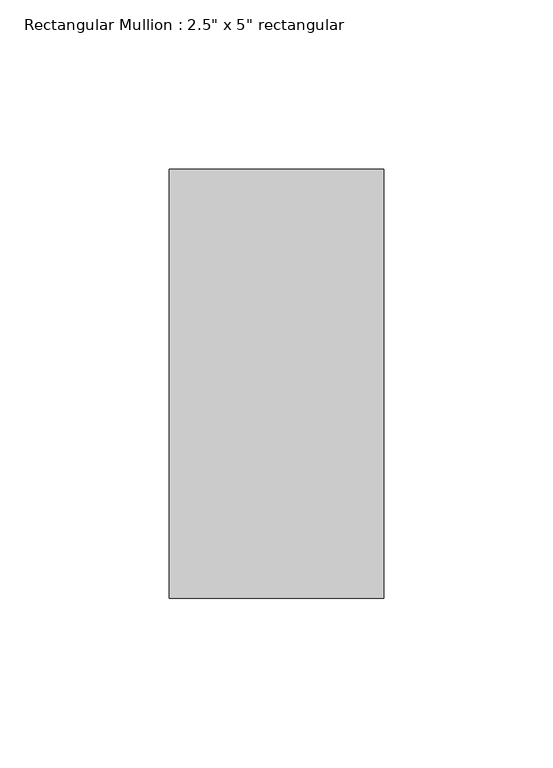
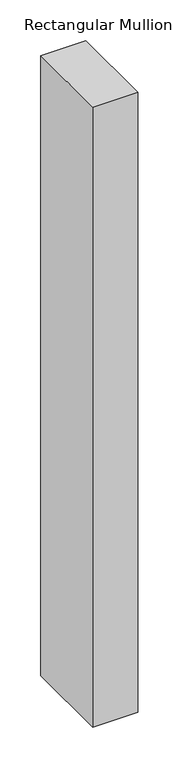
"""IFC4 building model written with IfcOpenShell, lengths in millimetres: member geometry."""

from ifc_helpers import new_model, si_unit, frame, origin, place, context, project, spatial, polyline, outline, extrude, source, transform, mapped, element, save


def member_d3800c19(model_context):
    return source(origin(), model_context, "Body", "SweptSolid", [
        extrude(outline(polyline([(0.0, 63.5), (0.0, -63.5), (-63.5, -63.5), (-63.5, 63.5), (0.0, 63.5)])), frame((0.0, 0.0, -925.9054943), z_axis=(0.0, 0.0, 1.0), x_axis=(1.0, 0.0, 0.0)), (0.0, 0.0, 1.0), 925.9054943),
    ])


if __name__ == "__main__":
    model = new_model("IFC4")
    model_context = context("Model", 3, world=origin())
    ifc_project = project(units=[si_unit("LENGTHUNIT", "METRE", prefix="MILLI")], contexts=[model_context])
    site = spatial("IfcSite", under=ifc_project)
    building = spatial("IfcBuilding", under=site)
    placement = place(None, origin())
    member_shape = member_d3800c19(model_context)
    element("IfcMember", 1, ObjectType="Rectangular Mullion : 2.5\" x 5\" rectangular", at=placement, inside=building, context=model_context, shape_type="MappedRepresentation", body=[
        mapped(member_shape, transform((0.0, 0.0, 0.0), x_axis=(1.0, 0.0, 0.0), y_axis=(0.0, 1.0, 0.0), z_axis=(0.0, 0.0, 1.0))),
    ])
    save(model, "model.ifc")

# Revit data of these elements
# Type "Rectangular Mullion : 2.5\" x 5\" rectangular"
#   built-in parameter 1007304 = 0.416667 (stored number, unit not read)
#   built-in parameter 1007301 = 0.104167 (stored number, unit not read)
#   built-in parameter 1007300 = 0.104167 (stored number, unit not read)
# Element 1 (IfcMember, "Rectangular Mullion : 2.5\" x 5\" rectangular")
#   Materials on its faces: "Aluminum"
# Materials
#   "Aluminum": class "Metal", colour RGB 247 247 247, transparency 0, Description = "Aluminum 6061", Cost = 0
